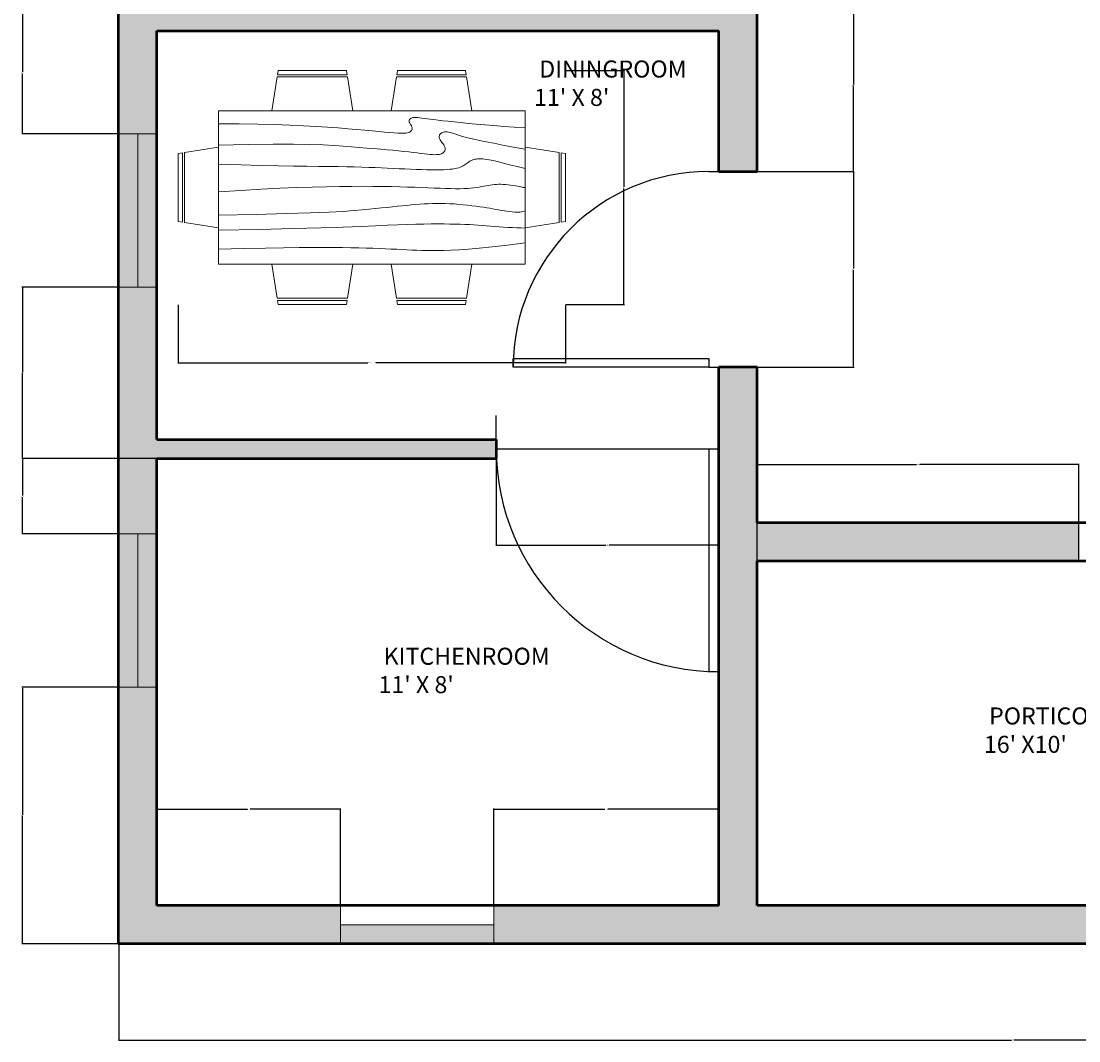
# Model space of a CAD drawing. Units: inches. Extents: x 7 to 493, y -11 to 454.
# Tile 1 of 4: x 7 to 255, y -11 to 228. Entities that reach past the tile are written whole.
import ezdxf

# ---------------------------------------------------------------- set-up
doc = ezdxf.new("R2010")
doc.units = ezdxf.units.IN
doc.header["$MEASUREMENT"] = 0
for name, color, linetype, lineweight in [('A-ANNO-DIMS', 2, 'Continuous', 18), ('A-AREA-IDEN', 7, 'Continuous', 25), ('A-WALL', 7, 'Continuous', 50), ('doors', 40, 'Continuous', 25), ('furniture', 220, 'Continuous', 18), ('window', 30, 'Continuous', 18)]:
    doc.layers.add(name, color=color, linetype=linetype, lineweight=lineweight)
doc.layers.add('A-WALL-PATT', color=251, linetype='Continuous', lineweight=13, true_color=0x636466)
doc.styles.get("Standard").update_dxf_attribs({"font": 'arial.ttf'})
doc.dimstyles.get("Standard").update_dxf_attribs({"dimtxt": 0.18, "dimasz": 0.18, "dimexe": 0.18, "dimexo": 0.0625, "dimgap": 0.09, "dimtad": 0, "dimtih": 1, "dimtoh": 1, "dimdec": 4, "dimzin": 0, "dimdsep": 46, "dimtxsty": 'Standard', "dimcen": 0.09, "dimadec": 0, "dimazin": 0, "dimtfac": 1, "dimtdec": 4, "dimtofl": 0, "dimtmove": 0, "dimatfit": 3, "dimfxl": 1, "dimtolj": 1, "dimtzin": 0, "dimarcsym": 0})

# ---------------------------------------------------------------- blocks, each defined once
blk = doc.blocks.new('Dining Set - 36 x 72 in.')
for p, q in [((-22, 27.5), (-22.1562, 26.50042)), ((-22, 27.5), (-6, 27.5)), ((-5.8437, 26.49966), (-6, 27.5)), ((6, 27.5), (5.8438, 26.50042)), ((6, 27.5), (22, 27.5)), ((22.1563, 26.49966), (22, 27.5)), ((-22.2343, 26.00059), (-23.4847, 17.99762)), ((-22.2304, 26), (-5.7608, 26)), ((-5.8416, 26.5), (-22.1534, 26.5)), ((-4.5152, 17.99762), (-5.7655, 25.99926)), ((5.7657, 26.00059), (4.5153, 17.99762)), ((5.7696, 26), (22.2392, 26)), ((22.1584, 26.5), (5.8466, 26.5)), ((23.4848, 17.99762), (22.2345, 25.99926)), ((36, 18), (-36, 18)), ((-36, 18), (-36, -18)), ((36, -18), (36, 18)), ((-45.5, 8), (-44.5004, 8.15617)), ((-45.5, 8), (-45.5, -8)), ((-44.5, -8.15843), (-44.5, 8.15338)), ((-44.0006, 8.23428), (-35.9976, 9.48474)), ((-44, 8.23041), (-44, -8.23915)), ((44.0006, 8.23428), (35.9976, 9.48474)), ((44, 8.23041), (44, -8.23915)), ((44.5, -8.15843), (44.5, 8.15338)), ((45.5, 8), (44.5005, 8.15617)), ((45.5, 8), (45.5, -8)), ((-44.4997, -8.15631), (-45.5, -8)), ((-35.9976, -9.48476), (-43.9993, -8.2345)), ((35.9976, -9.48476), (43.9993, -8.2345)), ((44.4997, -8.15631), (45.5, -8)), ((-36, -18), (36, -18)), ((-22.2343, -26.0006), (-23.4847, -17.99762)), ((-4.5152, -17.99762), (-5.7655, -25.99928)), ((5.7657, -26.0006), (4.5153, -17.99762)), ((23.4848, -17.99762), (22.2345, -25.99928)), ((-22.2304, -26), (-5.7608, -26)), ((-22, -27.5), (-22.1562, -26.50044)), ((-5.8416, -26.5), (-22.1534, -26.5)), ((-5.8437, -26.49967), (-6, -27.5)), ((5.7696, -26), (22.2392, -26)), ((6, -27.5), (5.8438, -26.50044)), ((22.1584, -26.5), (5.8466, -26.5)), ((22.1563, -26.49967), (22, -27.5)), ((-22, -27.5), (-6, -27.5)), ((6, -27.5), (22, -27.5))]:
    blk.add_line(p, q)
for points in [[(-36, 15), (-31.1772, 14.97754), (-26.8079, 14.91406), (-22.8538, 14.81543), (-19.276, 14.6875), (-16.0362, 14.53613), (-13.0957, 14.36718), (-10.4159, 14.18652), (-7.9583, 14), (-5.6904, 13.81315), (-3.6035, 13.63021), (-1.6954, 13.45508), (0.0365, 13.29166), (1.5945, 13.14388), (2.9811, 13.01562), (4.1988, 12.9108), (5.25, 12.83333), (6.1393, 12.78613), (6.8802, 12.76823), (7.4883, 12.77767), (7.9792, 12.8125), (8.3685, 12.87077), (8.6719, 12.95052), (8.9049, 13.0498), (9.0833, 13.16666), (9.2205, 13.29899), (9.3216, 13.44401), (9.3895, 13.59879), (9.4271, 13.76041), (9.4373, 13.92594), (9.4232, 14.09245), (9.3875, 14.257), (9.3333, 14.41666), (9.2638, 14.56917), (9.1836, 14.71484), (9.0975, 14.85465), (9.0104, 14.98958), (8.9272, 15.1206), (8.8529, 15.2487), (8.7922, 15.37483), (8.75, 15.5), (8.7305, 15.62467), (8.7344, 15.74739), (8.7617, 15.86621), (8.8125, 15.97916), (8.8867, 16.08431), (8.9844, 16.17968), (9.1055, 16.26334), (9.25, 16.33333), (9.4189, 16.38802), (9.6172, 16.42708), (9.8506, 16.45052), (10.125, 16.45833), (10.4463, 16.45052), (10.8203, 16.42708), (11.2529, 16.38802), (11.75, 16.33333), (12.3184, 16.26318), (12.9694, 16.17838), (13.7151, 16.07991), (14.5677, 15.96875), (15.5395, 15.84586), (16.6426, 15.71224), (17.8893, 15.56884), (19.2917, 15.41666), (20.859, 15.25667), (22.5879, 15.08984), (24.4721, 14.91715), (26.5052, 14.73958), (28.6809, 14.5581), (30.9929, 14.3737), (33.4347, 14.18733), (36, 14)], [(-36, 10), (-28.9766, 10.14274), (-23.1725, 10.20442), (-18.4241, 10.19775), (-14.5677, 10.13541), (-11.4399, 10.03011), (-8.877, 9.89453), (-6.7154, 9.74137), (-4.7917, 9.58333), (-2.9698, 9.43082), (-1.2246, 9.28515), (0.4415, 9.14534), (2.026, 9.01041), (3.5266, 8.87939), (4.9408, 8.7513), (6.266, 8.62516), (7.5, 8.5), (8.6411, 8.37549), (9.6914, 8.2539), (10.6538, 8.13818), (11.5312, 8.03125), (12.3267, 7.93603), (13.043, 7.85547), (13.6831, 7.79248), (14.25, 7.75), (14.7471, 7.7303), (15.1797, 7.73307), (15.5537, 7.75732), (15.875, 7.80208), (16.1494, 7.86637), (16.3828, 7.94922), (16.5811, 8.04964), (16.75, 8.16666), (16.8944, 8.29915), (17.0143, 8.44531), (17.1089, 8.60319), (17.1771, 8.77083), (17.218, 8.94629), (17.2305, 9.1276), (17.2137, 9.31282), (17.1667, 9.5), (17.0895, 9.6875), (16.987, 9.875), (16.8649, 10.0625), (16.7292, 10.25), (16.5856, 10.4375), (16.4401, 10.625), (16.2985, 10.8125), (16.1667, 11), (16.05, 11.18733), (15.9518, 11.3737), (15.8752, 11.5581), (15.8229, 11.73958), (15.798, 11.91715), (15.8034, 12.08984), (15.842, 12.25667), (15.9167, 12.41666), (16.0295, 12.56836), (16.1784, 12.70833), (16.3605, 12.83268), (16.5729, 12.9375), (16.8127, 13.01888), (17.0768, 13.07291), (17.3625, 13.0957), (17.6667, 13.08333), (17.9894, 13.03312), (18.3418, 12.94726), (18.7382, 12.82918), (19.1927, 12.68229), (19.7195, 12.51001), (20.3327, 12.31575), (21.0465, 12.10294), (21.875, 11.875), (22.8357, 11.63354), (23.959, 11.37304), (25.2786, 11.08618), (26.8282, 10.76562), (28.6414, 10.40405), (30.752, 9.99414), (33.1936, 9.52856), (36, 9)], [(-36, 5.5), (-30.7157, 5.3348), (-26.069, 5.20963), (-21.9946, 5.11767), (-18.4271, 5.05208), (-15.3009, 5.00602), (-12.5508, 4.97265), (-10.1112, 4.94515), (-7.9167, 4.91666), (-5.909, 4.88167), (-4.0586, 4.83984), (-2.3429, 4.79215), (-0.7396, 4.73958), (0.7739, 4.6831), (2.22, 4.6237), (3.6213, 4.56233), (5, 4.5), (6.373, 4.43782), (7.7344, 4.3776), (9.0723, 4.32129), (10.375, 4.27083), (11.6309, 4.22819), (12.8281, 4.19531), (13.9551, 4.17415), (15, 4.16666), (15.954, 4.17448), (16.819, 4.19791), (17.6001, 4.23698), (18.3021, 4.29166), (18.9299, 4.36198), (19.4883, 4.44791), (19.9823, 4.54948), (20.4167, 4.66666), (20.7969, 4.79899), (21.1302, 4.94401), (21.4245, 5.09879), (21.6875, 5.26041), (21.9271, 5.42594), (22.1511, 5.59245), (22.3672, 5.757), (22.5834, 5.91666), (22.8065, 6.06868), (23.0404, 6.21093), (23.2879, 6.34147), (23.5521, 6.45833), (23.8358, 6.55957), (24.142, 6.64323), (24.4735, 6.70735), (24.8334, 6.75), (25.2235, 6.76969), (25.642, 6.76692), (26.0858, 6.74267), (26.5521, 6.69791), (27.0379, 6.63362), (27.5404, 6.55078), (28.0565, 6.45036), (28.5834, 6.33333), (29.1242, 6.19987), (29.7071, 6.04687), (30.3661, 5.87044), (31.1354, 5.66666), (32.0493, 5.43164), (33.142, 5.16146), (34.4475, 4.85221), (36, 4.5)], [(-36, -1), (-30.7915, -0.6591), (-26.0195, -0.38216), (-21.6519, -0.16284), (-17.6563, 0.00521), (-14.0005, 0.12833), (-10.6523, 0.21289), (-7.5796, 0.26522), (-4.75, 0.29166), (-2.134, 0.29793), (0.2878, 0.28711), (2.5317, 0.26163), (4.6146, 0.22396), (6.5529, 0.17651), (8.3633, 0.12174), (10.0623, 0.06209), (11.6667, 0), (13.1899, -0.06201), (14.6341, -0.1211), (15.9982, -0.17432), (17.2813, -0.21875), (18.4823, -0.25147), (19.6003, -0.26953), (20.6343, -0.27002), (21.5834, -0.25), (22.4481, -0.20768), (23.2357, -0.14584), (23.9549, -0.06836), (24.6146, 0.02083), (25.2235, 0.11784), (25.7904, 0.21875), (26.3241, 0.31966), (26.8334, 0.41666), (27.3265, 0.50618), (27.8099, 0.58593), (28.2894, 0.65397), (28.7709, 0.70833), (29.2601, 0.74707), (29.763, 0.76823), (30.2855, 0.76985), (30.8334, 0.75), (31.4088, 0.70784), (31.9994, 0.64713), (32.589, 0.57275), (33.1615, 0.48958), (33.7008, 0.4025), (34.1908, 0.3164), (34.6153, 0.23616), (34.9584, 0.16666), (35.2099, 0.11165), (35.3848, 0.07031), (35.504, 0.04069), (35.5886, 0.02083), (35.6594, 0.00879), (35.7377, 0.0026), (35.8442, 0.00032), (36, 0)], [(-36, -6.5), (-27.1843, -6.31267), (-20.084, -6.1263), (-14.469, -5.9419), (-10.1094, -5.76042), (-6.7752, -5.58285), (-4.2363, -5.41016), (-2.2629, -5.24333), (-0.625, -5.08334), (0.8708, -4.93099), (2.2715, -4.78646), (3.5872, -4.64974), (4.8281, -4.52084), (6.0046, -4.39974), (7.127, -4.28646), (8.2053, -4.18099), (9.25, -4.08334), (10.2705, -3.99382), (11.2734, -3.91407), (12.2647, -3.84603), (13.25, -3.79167), (14.2354, -3.75293), (15.2266, -3.73177), (16.2295, -3.73015), (17.25, -3.75), (18.2912, -3.79248), (19.3451, -3.85547), (20.4009, -3.93604), (21.4479, -4.03125), (22.4754, -4.13819), (23.4727, -4.25391), (24.4289, -4.37549), (25.3334, -4.5), (26.1785, -4.62492), (26.9694, -4.74935), (27.7145, -4.87281), (28.4219, -4.99479), (29.1, -5.11483), (29.7572, -5.23242), (30.4016, -5.34709), (31.0417, -5.45834), (31.6837, -5.56437), (32.3262, -5.65821), (32.9658, -5.73153), (33.599, -5.77604), (34.2224, -5.78345), (34.8327, -5.74545), (35.4264, -5.65373), (36, -5.5)], [(-36, -10), (-26.4022, -9.81299), (-18.4675, -9.62891), (-11.9839, -9.45069), (-6.7396, -9.28125), (-2.5226, -9.12354), (0.8789, -8.98047), (3.6769, -8.85498), (6.0833, -8.75), (8.2767, -8.66765), (10.3021, -8.60677), (12.1712, -8.56543), (13.8958, -8.54167), (15.4876, -8.53353), (16.9583, -8.53907), (18.3197, -8.55632), (19.5834, -8.58334), (20.7616, -8.61841), (21.8685, -8.66081), (22.9188, -8.71004), (23.9271, -8.76563), (24.9081, -8.82707), (25.8763, -8.89388), (26.8465, -8.96558), (27.8334, -9.04167), (28.8474, -9.12118), (29.8828, -9.20117), (30.93, -9.27824), (31.9792, -9.34896), (33.0205, -9.40991), (34.0443, -9.45768), (35.0407, -9.48885), (36, -9.5)], [(-36, -14.5), (-30.0881, -14.33513), (-25.0332, -14.21224), (-20.7312, -14.12647), (-17.0781, -14.07292), (-13.97, -14.04671), (-11.3027, -14.04297), (-8.9724, -14.05681), (-6.875, -14.08334), (-4.9224, -14.11833), (-3.0905, -14.16016), (-1.3709, -14.20785), (0.2448, -14.26042), (1.7647, -14.3169), (3.1973, -14.3763), (4.5507, -14.43767), (5.8333, -14.5), (7.0554, -14.5621), (8.235, -14.62175), (9.3922, -14.67652), (10.5469, -14.72396), (11.7192, -14.76164), (12.929, -14.78711), (14.1965, -14.79794), (15.5417, -14.79167), (16.9933, -14.76424), (18.6152, -14.70508), (20.4804, -14.60197), (22.6615, -14.44271), (25.2312, -14.21509), (28.2624, -13.9069), (31.8277, -13.50594), (36, -13)]]:
    blk.add_lwpolyline(points)
blk = doc.blocks.new('*U4')
for p, q in [((0, 0), (0, -6)), ((40, 0), (40, -6))]:
    blk.add_line(p, q)
blk.add_lwpolyline([(0, 0), (0, 40), (1.75, 40), (1.75, 0)], close=True)
blk.add_arc((0, 0), 40, 0, 90)
blk = doc.blocks.new('*U8')
for p, q in [((-40, 0), (-40, 6)), ((0, 0), (0, 6))]:
    blk.add_line(p, q)
blk.add_lwpolyline([(0, 0), (0, -40), (-1.75, -40), (-1.75, 0)], close=True)
blk.add_arc((0, 0), 40, 180, 270)
blk = doc.blocks.new('WIN-36IN')
for p, q in [((0, 0), (0, 9)), ((0, 9), (36, 9)), ((36, 9), (36, 0)), ((36, 9), (36, 4.5)), ((36, 4.5), (0, 4.5)), ((36, 0), (0, 0))]:
    blk.add_line(p, q)
blk = doc.blocks.new('*D20')
at = {"layer": 'A-ANNO-DIMS', "color": 0, "lineweight": -2, "transparency": 16777216}
for p, q in [((43.79, 161.58), (43.79, 147.81)), ((134.79, 161.58), (134.79, 147.81)), ((43.97, 147.99), (88.34, 147.99)), ((134.61, 147.99), (90.25, 147.99))]:
    blk.add_line(p, q, dxfattribs=at)
at = {"layer": 'A-ANNO-DIMS', "color": 0, "transparency": 16777216}
for points in [[(43.97, 148.02), (43.97, 147.96), (43.79, 147.99)], [(134.61, 148.02), (134.61, 147.96), (134.79, 147.99)]]:
    blk.add_solid(points, dxfattribs=at)
at = {"layer": 'Defpoints', "color": 0, "transparency": 16777216}
for p in [(43.79, 161.64), (134.79, 161.64), (134.79, 147.99)]:
    blk.add_point(p, dxfattribs=at)
at = {"layer": 'A-ANNO-DIMS', "color": 0, "transparency": 16777216, "insert": (89.29, 147.99), "char_height": 0.18, "attachment_point": 5}
blk.add_mtext('\\A1;DINING SET 91', dxfattribs=at)
blk = doc.blocks.new('*D21')
at = {"layer": 'A-ANNO-DIMS', "color": 0, "lineweight": -2, "transparency": 16777216}
for p, q in [((134.86, 216.64), (148.62, 216.64)), ((148.44, 216.46), (148.44, 189.32)), ((148.44, 161.82), (148.44, 188.96)), ((134.86, 161.64), (148.62, 161.64))]:
    blk.add_line(p, q, dxfattribs=at)
at = {"layer": 'A-ANNO-DIMS', "color": 0, "transparency": 16777216}
for points in [[(148.41, 216.46), (148.47, 216.46), (148.44, 216.64)], [(148.41, 161.82), (148.47, 161.82), (148.44, 161.64)]]:
    blk.add_solid(points, dxfattribs=at)
at = {"layer": 'Defpoints', "color": 0, "transparency": 16777216}
for p in [(134.79, 216.64), (148.44, 216.64), (134.79, 161.64)]:
    blk.add_point(p, dxfattribs=at)
at = {"layer": 'A-ANNO-DIMS', "color": 0, "transparency": 16777216, "insert": (148.44, 189.14), "char_height": 0.18, "attachment_point": 5}
blk.add_mtext('\\A1;55', dxfattribs=at)
blk = doc.blocks.new('*D22')
at = {"layer": 'A-ANNO-DIMS', "color": 0, "lineweight": -2, "transparency": 16777216}
for p, q in [((29.81, 11.42), (29.81, -11.29)), ((449.81, 11.42), (449.81, -11.29)), ((29.99, -11.11), (239.51, -11.11)), ((449.63, -11.11), (240.1, -11.11))]:
    blk.add_line(p, q, dxfattribs=at)
at = {"layer": 'A-ANNO-DIMS', "color": 0, "transparency": 16777216}
for points in [[(29.99, -11.08), (29.99, -11.14), (29.81, -11.11)], [(449.63, -11.08), (449.63, -11.14), (449.81, -11.11)]]:
    blk.add_solid(points, dxfattribs=at)
at = {"layer": 'Defpoints', "color": 0, "transparency": 16777216}
for p in [(29.81, 11.49), (449.81, 11.49), (449.81, -11.11)]:
    blk.add_point(p, dxfattribs=at)
at = {"layer": 'A-ANNO-DIMS', "color": 0, "transparency": 16777216, "insert": (239.81, -11.11), "char_height": 0.18, "attachment_point": 5}
blk.add_mtext('\\A1;420', dxfattribs=at)
blk = doc.blocks.new('*D30')
at = {"layer": 'A-ANNO-DIMS', "color": 0, "lineweight": -2, "transparency": 16777216}
for p, q in [((29.74, 71.77), (7.03, 71.77)), ((7.21, 71.59), (7.21, 41.81)), ((7.21, 11.67), (7.21, 41.45)), ((29.74, 11.49), (7.03, 11.49))]:
    blk.add_line(p, q, dxfattribs=at)
at = {"layer": 'A-ANNO-DIMS', "color": 0, "transparency": 16777216}
for points in [[(7.18, 71.59), (7.24, 71.59), (7.21, 71.77)], [(7.18, 11.67), (7.24, 11.67), (7.21, 11.49)]]:
    blk.add_solid(points, dxfattribs=at)
at = {"layer": 'Defpoints', "color": 0, "transparency": 16777216}
for p in [(7.21, 71.77), (29.81, 71.77), (29.81, 11.49)]:
    blk.add_point(p, dxfattribs=at)
at = {"layer": 'A-ANNO-DIMS', "color": 0, "transparency": 16777216, "insert": (7.21, 41.63), "char_height": 0.18, "attachment_point": 5}
blk.add_mtext('\\A1;60.29', dxfattribs=at)
blk = doc.blocks.new('*D31')
at = {"layer": 'A-ANNO-DIMS', "color": 0, "lineweight": -2, "transparency": 16777216}
for p, q in [((38.74, 125.49), (7.03, 125.49)), ((7.21, 125.31), (7.21, 116.81)), ((7.21, 107.95), (7.21, 116.45)), ((29.74, 107.77), (7.03, 107.77))]:
    blk.add_line(p, q, dxfattribs=at)
at = {"layer": 'A-ANNO-DIMS', "color": 0, "transparency": 16777216}
for points in [[(7.18, 125.31), (7.24, 125.31), (7.21, 125.49)], [(7.18, 107.95), (7.24, 107.95), (7.21, 107.77)]]:
    blk.add_solid(points, dxfattribs=at)
at = {"layer": 'Defpoints', "color": 0, "transparency": 16777216}
for p in [(7.21, 125.49), (38.81, 125.49), (29.81, 107.77)]:
    blk.add_point(p, dxfattribs=at)
at = {"layer": 'A-ANNO-DIMS', "color": 0, "transparency": 16777216, "insert": (7.21, 116.63), "char_height": 0.18, "attachment_point": 5}
blk.add_mtext('\\A1;17.71', dxfattribs=at)
blk = doc.blocks.new('*D32')
at = {"layer": 'A-ANNO-DIMS', "color": 0, "lineweight": -2, "transparency": 16777216}
for p, q in [((29.74, 165.76), (7.03, 165.76)), ((7.21, 165.58), (7.21, 145.81)), ((7.21, 125.67), (7.21, 145.44)), ((38.74, 125.49), (7.03, 125.49))]:
    blk.add_line(p, q, dxfattribs=at)
at = {"layer": 'A-ANNO-DIMS', "color": 0, "transparency": 16777216}
for points in [[(7.18, 165.58), (7.24, 165.58), (7.21, 165.76)], [(7.18, 125.67), (7.24, 125.67), (7.21, 125.49)]]:
    blk.add_solid(points, dxfattribs=at)
at = {"layer": 'Defpoints', "color": 0, "transparency": 16777216}
for p in [(7.21, 165.76), (29.81, 165.76), (38.81, 125.49)]:
    blk.add_point(p, dxfattribs=at)
at = {"layer": 'A-ANNO-DIMS', "color": 0, "transparency": 16777216, "insert": (7.21, 145.63), "char_height": 0.18, "attachment_point": 5}
blk.add_mtext('\\A1;40.28', dxfattribs=at)
blk = doc.blocks.new('*D33')
at = {"layer": 'A-ANNO-DIMS', "color": 0, "lineweight": -2, "transparency": 16777216}
for p, q in [((38.74, 230.49), (7.03, 230.49)), ((7.21, 230.31), (7.21, 216.31)), ((7.21, 201.94), (7.21, 215.94)), ((29.74, 201.76), (7.03, 201.76))]:
    blk.add_line(p, q, dxfattribs=at)
at = {"layer": 'A-ANNO-DIMS', "color": 0, "transparency": 16777216}
for points in [[(7.18, 230.31), (7.24, 230.31), (7.21, 230.49)], [(7.18, 201.94), (7.24, 201.94), (7.21, 201.76)]]:
    blk.add_solid(points, dxfattribs=at)
at = {"layer": 'Defpoints', "color": 0, "transparency": 16777216}
for p in [(7.21, 230.49), (38.81, 230.49), (29.81, 201.76)]:
    blk.add_point(p, dxfattribs=at)
at = {"layer": 'A-ANNO-DIMS', "color": 0, "transparency": 16777216, "insert": (7.21, 216.13), "char_height": 0.18, "attachment_point": 5}
blk.add_mtext('\\A1;28.72', dxfattribs=at)
blk = doc.blocks.new('*D43')
at = {"layer": 'A-ANNO-DIMS', "color": 0, "lineweight": -2, "transparency": 16777216}
for p, q in [((38.81, 20.55), (38.81, 43.27)), ((38.99, 43.09), (60.04, 43.09)), ((81.72, 43.09), (60.66, 43.09)), ((81.9, 20.55), (81.9, 43.27))]:
    blk.add_line(p, q, dxfattribs=at)
at = {"layer": 'A-ANNO-DIMS', "color": 0, "transparency": 16777216}
for points in [[(38.99, 43.12), (38.99, 43.06), (38.81, 43.09)], [(81.72, 43.12), (81.72, 43.06), (81.9, 43.09)]]:
    blk.add_solid(points, dxfattribs=at)
at = {"layer": 'Defpoints', "color": 0, "transparency": 16777216}
for p in [(81.9, 43.09), (38.81, 20.49), (81.9, 20.49)]:
    blk.add_point(p, dxfattribs=at)
at = {"layer": 'A-ANNO-DIMS', "color": 0, "transparency": 16777216, "insert": (60.35, 43.09), "char_height": 0.18, "attachment_point": 5}
blk.add_mtext('\\A1;43.1', dxfattribs=at)
blk = doc.blocks.new('*D44')
at = {"layer": 'A-ANNO-DIMS', "color": 0, "lineweight": -2, "transparency": 16777216}
for p, q in [((117.9, 20.55), (117.9, 43.27)), ((118.08, 43.09), (144.03, 43.09)), ((170.63, 43.09), (144.68, 43.09)), ((170.81, 20.55), (170.81, 43.27))]:
    blk.add_line(p, q, dxfattribs=at)
at = {"layer": 'A-ANNO-DIMS', "color": 0, "transparency": 16777216}
for points in [[(118.08, 43.12), (118.08, 43.06), (117.9, 43.09)], [(170.63, 43.12), (170.63, 43.06), (170.81, 43.09)]]:
    blk.add_solid(points, dxfattribs=at)
at = {"layer": 'Defpoints', "color": 0, "transparency": 16777216}
for p in [(170.81, 43.09), (117.9, 20.49), (170.81, 20.49)]:
    blk.add_point(p, dxfattribs=at)
at = {"layer": 'A-ANNO-DIMS', "color": 0, "transparency": 16777216, "insert": (144.35, 43.09), "char_height": 0.18, "attachment_point": 5}
blk.add_mtext('\\A1;52.9', dxfattribs=at)
blk = doc.blocks.new('*D45')
at = {"layer": 'A-ANNO-DIMS', "color": 0, "lineweight": -2, "transparency": 16777216}
for p, q in [((179.81, 101.55), (179.81, 124.27)), ((255.37, 101.55), (255.37, 124.27)), ((179.99, 124.09), (217.19, 124.09)), ((255.19, 124.09), (217.98, 124.09))]:
    blk.add_line(p, q, dxfattribs=at)
at = {"layer": 'A-ANNO-DIMS', "color": 0, "transparency": 16777216}
for points in [[(179.99, 124.12), (179.99, 124.06), (179.81, 124.09)], [(255.19, 124.12), (255.19, 124.06), (255.37, 124.09)]]:
    blk.add_solid(points, dxfattribs=at)
at = {"layer": 'Defpoints', "color": 0, "transparency": 16777216}
for p in [(255.37, 124.09), (179.81, 101.49), (255.37, 101.49)]:
    blk.add_point(p, dxfattribs=at)
at = {"layer": 'A-ANNO-DIMS', "color": 0, "transparency": 16777216, "insert": (217.59, 124.09), "char_height": 0.18, "attachment_point": 5}
blk.add_mtext('\\A1;75.56', dxfattribs=at)
blk = doc.blocks.new('*D50')
at = {"layer": 'A-ANNO-DIMS', "color": 0, "lineweight": -2, "transparency": 16777216}
for p, q in [((179.87, 192.92), (202.59, 192.92)), ((202.41, 192.74), (202.41, 170.13)), ((202.41, 147.16), (202.41, 169.77)), ((179.87, 146.98), (202.59, 146.98))]:
    blk.add_line(p, q, dxfattribs=at)
at = {"layer": 'A-ANNO-DIMS', "color": 0, "transparency": 16777216}
for points in [[(202.38, 192.74), (202.44, 192.74), (202.41, 192.92)], [(202.38, 147.16), (202.44, 147.16), (202.41, 146.98)]]:
    blk.add_solid(points, dxfattribs=at)
at = {"layer": 'Defpoints', "color": 0, "transparency": 16777216}
for p in [(179.81, 192.92), (179.81, 146.98), (202.41, 146.98)]:
    blk.add_point(p, dxfattribs=at)
at = {"layer": 'A-ANNO-DIMS', "color": 0, "transparency": 16777216, "insert": (202.41, 169.95), "char_height": 0.18, "attachment_point": 5}
blk.add_mtext('\\A1;45.94', dxfattribs=at)
blk = doc.blocks.new('*D51')
at = {"layer": 'A-ANNO-DIMS', "color": 0, "lineweight": -2, "transparency": 16777216}
for p, q in [((179.87, 233.49), (202.59, 233.49)), ((202.41, 233.31), (202.41, 213.38)), ((202.41, 193.1), (202.41, 213.02)), ((179.87, 192.92), (202.59, 192.92))]:
    blk.add_line(p, q, dxfattribs=at)
at = {"layer": 'A-ANNO-DIMS', "color": 0, "transparency": 16777216}
for points in [[(202.38, 233.31), (202.44, 233.31), (202.41, 233.49)], [(202.38, 193.1), (202.44, 193.1), (202.41, 192.92)]]:
    blk.add_solid(points, dxfattribs=at)
at = {"layer": 'Defpoints', "color": 0, "transparency": 16777216}
for p in [(179.81, 233.49), (179.81, 192.92), (202.41, 192.92)]:
    blk.add_point(p, dxfattribs=at)
at = {"layer": 'A-ANNO-DIMS', "color": 0, "transparency": 16777216, "insert": (202.41, 213.2), "char_height": 0.18, "attachment_point": 5}
blk.add_mtext('\\A1;40.57', dxfattribs=at)
blk = doc.blocks.new('*D52')
at = {"layer": 'A-ANNO-DIMS', "color": 0, "lineweight": -2, "transparency": 16777216}
for p, q in [((118.49, 127.67), (118.49, 104.96)), ((170.81, 127.67), (170.81, 104.96)), ((118.67, 105.14), (144.27, 105.14)), ((170.63, 105.14), (145.03, 105.14))]:
    blk.add_line(p, q, dxfattribs=at)
at = {"layer": 'A-ANNO-DIMS', "color": 0, "transparency": 16777216}
for points in [[(118.67, 105.17), (118.67, 105.11), (118.49, 105.14)], [(170.63, 105.17), (170.63, 105.11), (170.81, 105.14)]]:
    blk.add_solid(points, dxfattribs=at)
at = {"layer": 'Defpoints', "color": 0, "transparency": 16777216}
for p in [(118.49, 127.74), (170.81, 127.74), (118.49, 105.14)]:
    blk.add_point(p, dxfattribs=at)
at = {"layer": 'A-ANNO-DIMS', "color": 0, "transparency": 16777216, "insert": (144.65, 105.14), "char_height": 0.18, "attachment_point": 5}
blk.add_mtext('\\A1;52.31', dxfattribs=at)

msp = doc.modelspace()

# ---------------------------------------------------------------- hatches: boundary and pattern name
at = {"layer": 'A-WALL-PATT'}
h = msp.add_hatch(color=256, dxfattribs=at)
h.dxf.hatch_style = 1
h.paths.add_polyline_path([(29.8054, 11.4863), (449.8054, 11.4863), (449.8054, 431.4863), (29.8054, 431.4863)])
h.paths.add_polyline_path([(38.8054, 422.4863), (235.3054, 422.4863), (235.3054, 362.4863), (179.8054, 362.4863), (179.8054, 390.4863), (170.8054, 390.4863), (170.8054, 293.4863), (353.0513, 293.4863), (353.0513, 297.9863), (239.8054, 297.9863), (235.3054, 297.9863), (179.8054, 297.9863), (179.8054, 357.9863), (235.3054, 357.9863), (235.3054, 329.9863), (239.8054, 329.9863), (239.8054, 422.4863), (440.8054, 422.4863), (440.8054, 297.9863), (413.0513, 297.9863), (413.0513, 293.4863), (440.8054, 293.4863), (440.8054, 110.4863), (402.7135, 110.4863), (402.7135, 101.5532), (402.7135, 101.4863), (440.8054, 101.4863), (440.8054, 20.4863), (179.8054, 20.4863), (179.8054, 101.4863), (255.3658, 101.4863), (255.3658, 110.4863), (179.8054, 110.4863), (179.8054, 146.9794), (170.8054, 146.9794), (170.8054, 20.4863), (117.9037, 20.4863), (117.9037, 15.9863), (81.9037, 15.9863), (81.9037, 20.4863), (38.8054, 20.4863), (38.8054, 125.4863), (118.4942, 125.4863), (118.4942, 129.9863), (38.8054, 129.9863), (38.8054, 225.9863), (170.8054, 225.9863), (170.8054, 192.9161), (179.8054, 192.9161), (179.8054, 233.4863), (170.8054, 233.4863), (170.8054, 230.4863), (38.8054, 230.4863)], flags=16)
h.paths.add_polyline_path([(53.2938, 207.1427), (65.8095, 207.1427), (67.0594, 215.1427), (83.5282, 215.1427), (84.7782, 207.1427), (93.8095, 207.1427), (95.0594, 215.1427), (111.5282, 215.1427), (112.7782, 207.1427), (125.2938, 207.1427), (125.2938, 198.6271), (133.2938, 197.3771), (133.2938, 180.9083), (125.2938, 179.6583), (125.2938, 171.1427), (112.7782, 171.1427), (111.5282, 163.1427), (95.0594, 163.1427), (93.8095, 171.1427), (84.7782, 171.1427), (83.5282, 163.1427), (67.0594, 163.1427), (65.8095, 171.1427), (53.2938, 171.1427), (53.2938, 179.6583), (45.2938, 180.9083), (45.2938, 197.3771), (53.2938, 198.6271)], flags=0)
h.paths.add_polyline_path([(98.6154, 202.5867), (98.6833, 202.7415), (98.7209, 202.9031), (98.7311, 203.0686), (98.717, 203.2352), (98.6813, 203.3997), (98.6271, 203.5594), (98.5576, 203.7119), (98.4774, 203.8575), (98.3913, 203.9974), (98.2332, 204.2423), (98.1033, 204.4662), (98.0223, 204.7063), (98.0302, 204.9526), (98.1325, 205.1802), (98.329, 205.372), (98.3993, 205.406), (98.2782, 205.3224), (98.1805, 205.227), (98.1063, 205.1219), (98.0555, 205.0089), (98.0282, 204.8901), (98.0243, 204.7674), (98.0438, 204.6427), (98.086, 204.5175), (98.1467, 204.3914), (98.221, 204.2633), (98.3042, 204.1323), (98.4533, 203.9013), (98.6038, 203.6279), (98.7103, 203.3143), (98.7386, 202.9794), (98.6633, 202.6554)], flags=0)
h.paths.add_polyline_path([(67.2938, 216.6427), (83.2938, 216.6427), (83.45, 215.6427), (67.1375, 215.6427)], flags=0)
h.paths.add_polyline_path([(43.7938, 197.1427), (44.7938, 197.2989), (44.7938, 180.9864), (43.7938, 181.1427)], flags=0)
h.paths.add_polyline_path([(106.3833, 198.8302), (106.2808, 199.0177), (106.1587, 199.2052), (106.023, 199.3927), (105.8794, 199.5802), (105.6298, 199.9018), (105.4605, 200.1427), (105.3438, 200.33), (105.1938, 200.6147), (105.0892, 200.9776), (105.1, 201.3227), (105.1358, 201.3994), (105.0972, 201.2325), (105.0918, 201.0599), (105.1167, 200.8823), (105.169, 200.7008), (105.2456, 200.5164), (105.3438, 200.33), (105.4605, 200.1427), (105.5923, 199.9552), (105.7339, 199.7677), (105.8794, 199.5802), (106.1138, 199.2741), (106.3496, 198.9121)], flags=0)
h.paths.add_polyline_path([(124.5037, 189.2544), (124.6786, 189.213), (124.7978, 189.1834), (124.8824, 189.1635), (124.9532, 189.1515), (125.0583, 189.1432), (125.138, 189.143), (124.9529, 189.147), (124.7978, 189.1834), (124.5749, 189.2388)], flags=0)
h.paths.add_polyline_path([(95.2938, 216.6427), (111.2938, 216.6427), (111.45, 215.6427), (95.1375, 215.6427)], flags=0)
h.paths.add_polyline_path([(191.6785, 332.1221), (224.065, 332.1221), (224.065, 343.8649), (191.6785, 343.8649)], flags=8)
h.paths.add_polyline_path([(196.7522, 379.4931), (229.1387, 379.4931), (229.1387, 391.2359), (196.7522, 391.2359)], flags=8)
h.paths.add_polyline_path([(232.397, 56.3062), (260.115, 56.3062), (260.115, 68.0654), (232.397, 68.0654)], flags=8)
h.paths.add_polyline_path([(90.1783, 70.3293), (134.3492, 70.3293), (134.3492, 82.0885), (90.1783, 82.0885)], flags=8)
h.paths.add_polyline_path([(126.7274, 208.2711), (165.9297, 208.2711), (165.9297, 220.0303), (126.7274, 220.0303)], flags=8)
h.paths.add_polyline_path([(261.4741, 205.6105), (297.4786, 205.6105), (297.4786, 217.3697), (261.4741, 217.3697)], flags=8)
h.paths.add_polyline_path([(77.3838, 283.1969), (106.5561, 283.1969), (106.5561, 294.9561), (77.3838, 294.9561)], flags=8)
h.paths.add_polyline_path([(357.5163, 353.5423), (386.6886, 353.5423), (386.6886, 365.3015), (357.5163, 365.3015)], flags=8)

# ---------------------------------------------------------------- linework, layer by layer
at = {"layer": 'A-WALL'}
for p, q in [((179.8054, 192.9161), (179.8054, 233.4863)), ((38.8054, 225.9863), (170.8054, 225.9863)), ((38.8054, 129.9863), (38.8054, 225.9863)), ((170.8054, 192.9161), (170.8054, 225.9863)), ((170.8054, 192.9161), (179.8054, 192.9161)), ((170.8054, 20.4863), (170.8054, 146.9794)), ((179.8054, 146.9794), (170.8054, 146.9794)), ((179.8054, 110.4863), (179.8054, 146.9794)), ((38.8054, 129.9863), (118.4942, 129.9863)), ((118.4942, 129.9863), (118.4942, 125.4863)), ((38.8054, 125.4863), (118.4942, 125.4863)), ((38.8054, 20.4863), (38.8054, 125.4863)), ((179.8054, 110.4863), (330.7135, 110.4863)), ((179.8054, 101.4863), (330.7135, 101.4863)), ((179.8054, 20.4863), (179.8054, 101.4863)), ((170.8054, 20.4863), (38.8054, 20.4863)), ((440.8054, 20.4863), (179.8054, 20.4863))]:
    msp.add_line(p, q, dxfattribs=at)
msp.add_lwpolyline([(29.8054, 431.4863), (449.8054, 431.4863), (449.8054, 11.4863), (29.8054, 11.4863)], close=True, dxfattribs=at)
at = {"layer": 'doors'}
msp.add_line((118.4942, 127.7363), (170.8054, 127.7363), dxfattribs=at)

# ---------------------------------------------------------------- block references
at = {"layer": 'doors', "xscale": 1.148415726495933, "yscale": 1.148415726495933, "zscale": 1.148415726495933, "rotation": 90}
msp.add_blockref('*U4', (168.4149, 146.9794), dxfattribs=at)
at = {"layer": 'doors', "xscale": 1.307777551917458, "yscale": 1.307777551917458, "zscale": 1.307777551917458}
msp.add_blockref('*U8', (170.8054, 127.7363), dxfattribs=at)
at = {"layer": 'furniture'}
msp.add_blockref('Dining Set - 36 x 72 in.', (89.2938, 189.1427), dxfattribs=at)
at = {"layer": 'window', "extrusion": (0, 0, -1), "zscale": -1, "rotation": 269.9999999999984}
for p in [(-38.8057, 201.7638), (-38.8057, 107.7745)]:
    msp.add_blockref('WIN-36IN', p, dxfattribs=at)
at = {"layer": 'window'}
msp.add_blockref('WIN-36IN', (81.9039, 11.486), dxfattribs=at)

# ---------------------------------------------------------------- texts
at = {"layer": 'A-AREA-IDEN', "char_height": 0.2, "attachment_point": 1}
for s, insert in [("{\\H20x; DININGROOM\\P11' X 8'}", (127.3859, 218.9925)), ("{\\H20x; KITCHENROOM\\P11' X 8'}", (90.8368, 81.0508)), ("{\\H20x; PORTICO\\P16' X10'}", (233.0554, 67.0277))]:
    msp.add_mtext_dynamic_manual_height_columns(s, width=58.591086, gutter_width=1, heights=[0], dxfattribs=dict(at, insert=insert))

# ---------------------------------------------------------------- dimensions: what is measured, and where the dimension line sits
at = {"layer": 'A-ANNO-DIMS'}
for base, p1, p2, angle, override, picture, middle in [((202.4054, 192.9161), (179.8054, 233.4863), (179.8054, 192.9161), 270, {"dimdec": 2, "dimlfac": 1, "dimrnd": 0, "dimzin": 0, "dimdsep": 46, "dimlunit": 2}, '*D51', (202.4054, 213.2012)), ((7.2054, 230.4863), (29.8054, 201.764), (38.8054, 230.4863), 90, {"dimdec": 2, "dimlfac": 1, "dimrnd": 0, "dimzin": 0, "dimdsep": 46, "dimlunit": 2}, '*D33', (7.2054, 216.1252)), ((148.4438, 216.6427), (134.7938, 161.6427), (134.7938, 216.6427), 90, {"dimdec": 0, "dimlfac": 1, "dimrnd": 0, "dimzin": 0, "dimdsep": 46, "dimlunit": 2}, '*D21', (148.4438, 189.1427)), ((202.4054, 146.9794), (179.8054, 192.9161), (179.8054, 146.9794), 270, {"dimdec": 2, "dimlfac": 1, "dimrnd": 0, "dimzin": 0, "dimdsep": 46, "dimlunit": 2}, '*D50', (202.4054, 169.9478)), ((7.2054, 165.764), (38.8054, 125.4863), (29.8054, 165.764), 90, {"dimdec": 2, "dimlfac": 1, "dimrnd": 0, "dimzin": 0, "dimdsep": 46, "dimlunit": 2}, '*D32', (7.2054, 145.6252)), ((118.4942, 105.1363), (170.8054, 127.7363), (118.4942, 127.7363), 180, {"dimdec": 2, "dimlfac": 1, "dimrnd": 0, "dimzin": 0, "dimdsep": 46, "dimlunit": 2}, '*D52', (144.6498, 105.1363)), ((7.2054, 125.4863), (29.8054, 107.7747), (38.8054, 125.4863), 90, {"dimdec": 2, "dimlfac": 1, "dimrnd": 0, "dimzin": 0, "dimdsep": 46, "dimlunit": 2}, '*D31', (7.2054, 116.6305)), ((7.2054, 71.7747), (29.8054, 11.4863), (29.8054, 71.7747), 90, {"dimdec": 2, "dimlfac": 1, "dimrnd": 0, "dimzin": 0, "dimdsep": 46, "dimlunit": 2}, '*D30', (7.2054, 41.6305)), ((81.9037, 43.0863), (38.8054, 20.4863), (81.9037, 20.4863), 0, {"dimdec": 1, "dimlfac": 1, "dimrnd": 0, "dimzin": 0, "dimdsep": 46, "dimlunit": 2}, '*D43', (60.3545, 43.0863))]:
    dim = msp.add_linear_dim(base=base, p1=p1, p2=p2, angle=angle, dimstyle='Standard', override=override, dxfattribs=at)
    dim.commit()
    dim.dimension.update_dxf_attribs({"geometry": picture, "text_midpoint": middle})
dim = msp.add_linear_dim(base=(134.7938, 147.9927), p1=(43.7938, 161.6427), p2=(134.7938, 161.6427), text='DINING SET <>', dimstyle='Standard', override={"dimdec": 0, "dimlfac": 1, "dimrnd": 0, "dimzin": 0, "dimdsep": 46, "dimlunit": 2}, dxfattribs=at)
dim.commit()
dim.dimension.update_dxf_attribs({"geometry": '*D20', "text_midpoint": (89.2938, 147.9927)})
for base, p1, p2, override, picture, middle in [((255.3658, 124.0863), (179.8054, 101.4863), (255.3658, 101.4863), {"dimdec": 2, "dimlfac": 1, "dimrnd": 0, "dimzin": 0, "dimdsep": 46, "dimlunit": 2}, '*D45', (217.5856, 124.0863)), ((170.8054, 43.0863), (117.9037, 20.4863), (170.8054, 20.4863), {"dimdec": 1, "dimlfac": 1, "dimrnd": 0, "dimzin": 0, "dimdsep": 46, "dimlunit": 2}, '*D44', (144.3545, 43.0863)), ((449.8054, -11.1137), (29.8054, 11.4863), (449.8054, 11.4863), {"dimdec": 0, "dimlfac": 1, "dimrnd": 0, "dimzin": 0, "dimdsep": 46, "dimlunit": 2}, '*D22', (239.8054, -11.1137))]:
    dim = msp.add_linear_dim(base=base, p1=p1, p2=p2, dimstyle='Standard', override=override, dxfattribs=at)
    dim.commit()
    dim.dimension.update_dxf_attribs({"geometry": picture, "text_midpoint": middle})

doc.saveas('drawing.dxf')
